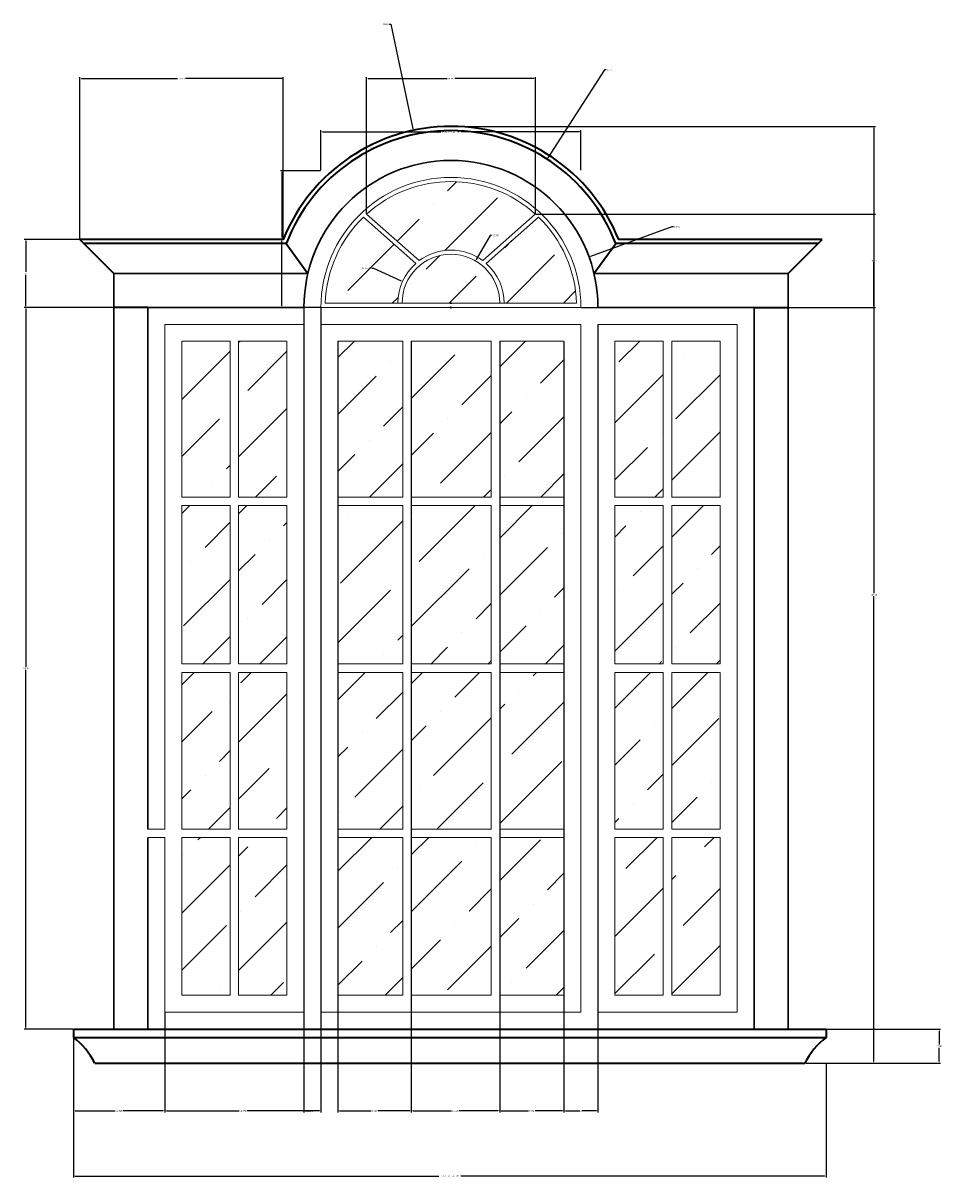
# Model space of a CAD drawing. Units: inches. Extents: x 386 to 708, y 151 to 489.
# Tile 3 of 4: x 386 to 494, y 353 to 489. Entities that reach past the tile are written whole.
import ezdxf

# ---------------------------------------------------------------- set-up
doc = ezdxf.new("R2010")
doc.units = ezdxf.units.IN
doc.header["$MEASUREMENT"] = 0
for name, color, linetype, lineweight in [('A-ANNO-DIMS', 2, 'Continuous', 18), ('A-GLAZ-FRAM', 4, 'Continuous', 30), ('A-GLAZ-PATT', 252, 'Continuous', 13), ('A-GLAZ-SASH', 4, 'Continuous', 18), ('A-GLAZ-SILL', 7, 'Continuous', 35), ('A-GLAZ-TRIM', 7, 'Continuous', 35)]:
    doc.layers.add(name, color=color, linetype=linetype, lineweight=lineweight)
doc.styles.get("Standard").update_dxf_attribs({"font": 'arial.ttf'})
doc.dimstyles.get("Standard").update_dxf_attribs({"dimtxt": 0.18, "dimasz": 0.18, "dimexe": 0.18, "dimexo": 0.0625, "dimgap": 0.09, "dimtad": 0, "dimtih": 1, "dimtoh": 1, "dimdec": 4, "dimzin": 0, "dimdsep": 46, "dimtxsty": 'Standard', "dimcen": 0.09, "dimadec": 0, "dimazin": 0, "dimtfac": 1, "dimtdec": 4, "dimtofl": 0, "dimtmove": 0, "dimatfit": 3, "dimfxl": 1, "dimtolj": 1, "dimtzin": 0, "dimarcsym": 0})

# ---------------------------------------------------------------- blocks, each defined once
blk = doc.blocks.new('WIN-SASH-2X4-L')
for p, q in [((9.69, 60.63), (9.69, 78.96)), ((10.69, 60.63), (10.69, 78.96)), ((4, 60.63), (9.69, 60.63)), ((10.69, 60.63), (16.38, 60.63)), ((4, 59.63), (9.69, 59.63)), ((9.69, 40.98), (9.69, 59.63)), ((10.69, 59.63), (16.38, 59.63)), ((10.69, 40.98), (10.69, 59.63)), ((4, 40.98), (9.69, 40.98)), ((10.69, 40.98), (16.38, 40.98)), ((4, 39.98), (9.69, 39.98)), ((9.69, 21.54), (9.69, 39.98)), ((10.69, 39.98), (16.38, 39.98)), ((10.69, 21.54), (10.69, 39.98)), ((0, 21.54), (2, 21.54)), ((0, 20.54), (2, 20.54)), ((4, 21.54), (9.69, 21.54)), ((4, 20.54), (9.69, 20.54)), ((9.69, 2), (9.69, 20.54)), ((10.69, 21.54), (16.38, 21.54)), ((10.69, 2), (10.69, 20.54)), ((10.69, 20.54), (16.38, 20.54))]:
    blk.add_line(p, q)
for points in [[(2, 20.54), (2, 0), (18.38, 0), (18.38, 80.96), (2, 80.96), (2, 21.54)], [(9.69, 78.96), (4, 78.96), (4, 60.63)], [(16.38, 60.63), (16.38, 78.96), (10.69, 78.96)], [(4, 59.63), (4, 40.98)], [(16.38, 40.98), (16.38, 59.63)], [(4, 39.98), (4, 21.54)], [(16.38, 21.54), (16.38, 39.98)], [(4, 20.54), (4, 2), (9.69, 2)], [(10.69, 2), (16.38, 2), (16.38, 20.54)]]:
    blk.add_lwpolyline(points)
blk = doc.blocks.new('WIN-SASH-2X4-R')
for p, q in [((7.69, 60.63), (7.69, 78.96)), ((8.69, 60.63), (8.69, 78.96)), ((2, 60.63), (7.69, 60.63)), ((8.69, 60.63), (14.38, 60.63)), ((2, 59.63), (7.69, 59.63)), ((7.69, 40.98), (7.69, 59.63)), ((8.69, 40.98), (8.69, 59.63)), ((8.69, 59.63), (14.38, 59.63)), ((2, 40.98), (7.69, 40.98)), ((8.69, 40.98), (14.38, 40.98)), ((2, 39.98), (7.69, 39.98)), ((7.69, 21.54), (7.69, 39.98)), ((8.69, 21.54), (8.69, 39.98)), ((8.69, 39.98), (14.38, 39.98)), ((2, 21.54), (7.69, 21.54)), ((2, 20.54), (7.69, 20.54)), ((7.69, 2), (7.69, 20.54)), ((8.69, 21.54), (14.38, 21.54)), ((8.69, 2), (8.69, 20.54)), ((8.69, 20.54), (14.38, 20.54))]:
    blk.add_line(p, q)
blk.add_lwpolyline([(0, 0), (16.38, 0), (16.38, 80.96), (0, 80.96)], close=True)
for points in [[(7.69, 78.96), (2, 78.96), (2, 60.63)], [(14.38, 60.63), (14.38, 78.96), (8.69, 78.96)], [(2, 59.63), (2, 40.98)], [(14.38, 40.98), (14.38, 59.63)], [(2, 39.98), (2, 21.54)], [(14.38, 21.54), (14.38, 39.98)], [(2, 20.54), (2, 2), (7.69, 2)], [(8.69, 2), (14.38, 2), (14.38, 20.54)]]:
    blk.add_lwpolyline(points)
blk = doc.blocks.new('WIN-SASH-3X4')
for p, q in [((9.62, 60.63), (9.62, 78.96)), ((10.62, 60.63), (10.62, 78.96)), ((20.04, 60.63), (20.04, 78.96)), ((21.04, 60.63), (21.04, 78.96)), ((2, 60.63), (9.62, 60.63)), ((10.62, 60.63), (20.04, 60.63)), ((21.04, 60.63), (28.6, 60.63)), ((21.04, 60.63), (28.6, 60.63)), ((2, 59.63), (9.62, 59.63)), ((9.62, 40.98), (9.62, 59.63)), ((10.62, 40.98), (10.62, 59.63)), ((10.62, 59.63), (20.04, 59.63)), ((20.04, 40.98), (20.04, 59.63)), ((21.04, 59.63), (28.6, 59.63)), ((21.04, 40.98), (21.04, 59.63)), ((21.04, 59.63), (28.6, 59.63)), ((2, 40.98), (9.62, 40.98)), ((10.62, 40.98), (20.04, 40.98)), ((21.04, 40.98), (28.6, 40.98)), ((21.04, 40.98), (28.6, 40.98)), ((2, 39.98), (9.62, 39.98)), ((9.62, 21.54), (9.62, 39.98)), ((10.62, 21.54), (10.62, 39.98)), ((10.62, 39.98), (20.04, 39.98)), ((20.04, 21.54), (20.04, 39.98)), ((21.04, 39.98), (28.6, 39.98)), ((21.04, 21.54), (21.04, 39.98)), ((21.04, 39.98), (28.6, 39.98)), ((2, 21.54), (9.62, 21.54)), ((2, 20.54), (9.62, 20.54)), ((9.62, 2), (9.62, 20.54)), ((10.62, 21.54), (20.04, 21.54)), ((10.62, 2), (10.62, 20.54)), ((10.62, 20.54), (20.04, 20.54)), ((20.04, 2), (20.04, 20.54)), ((21.04, 21.54), (28.6, 21.54)), ((21.04, 21.54), (28.6, 21.54)), ((21.04, 2), (21.04, 20.54)), ((21.04, 20.54), (28.6, 20.54)), ((21.04, 20.54), (28.6, 20.54))]:
    blk.add_line(p, q)
blk.add_lwpolyline([(30.6, 0), (30.6, 80.96), (0, 80.96), (0, 0)], close=True)
for points in [[(9.62, 78.96), (2, 78.96), (2, 60.63)], [(20.04, 78.96), (10.62, 78.96)], [(28.6, 60.63), (28.6, 78.96), (21.04, 78.96)], [(2, 59.63), (2, 40.98)], [(28.6, 40.98), (28.6, 59.63)], [(2, 39.98), (2, 21.54)], [(28.6, 21.54), (28.6, 39.98)], [(2, 20.54), (2, 2), (9.62, 2)], [(21.04, 2), (28.6, 2), (28.6, 20.54)], [(10.62, 2), (20.04, 2)]]:
    blk.add_lwpolyline(points)
blk = doc.blocks.new('WIN-FANLIGHT-RADIAL')
for p, q in [((11.55, 5.5), (5.37, 10.98)), ((19.05, 5.5), (25.23, 10.98)), ((11.16, 5.18), (5.01, 10.63)), ((19.44, 5.18), (25.6, 10.63))]:
    blk.add_line(p, q)
blk.add_lwpolyline([(30.6, 0), (0, 0, -1)], format="xyb", close=True)
for points in [[(5.37, 10.98, -0.385138), (25.23, 10.98, -0.385138)], [(25.6, 10.63, -0.194348), (30.09, 0.5), (0.51, 0.5, -0.194348), (5.01, 10.63)]]:
    blk.add_lwpolyline(points, format="xyb")
for radius, start, end in [(5.75, 0, 180), (6.25, 53.1161, 126.8839), (6.25, 131.5309, 180), (6.25, 0, 48.4691)]:
    blk.add_arc((15.3, 0.5), radius, start, end)
blk = doc.blocks.new('WIN-SILL-TRIPLE')
for p, q in [((0, 4), (88.59, 4)), ((0, 4), (0, 3)), ((0, 3), (88.59, 3)), ((88.59, 4), (88.59, 3)), ((2.5, 0), (86.09, 0))]:
    blk.add_line(p, q)
blk.add_lwpolyline([(4.75, 0), (84.1, 0)])
for centre, start, end in [((-4.74, -3.48), 25.6893, 53.8074), ((93.33, -3.48), 126.1926, 154.3107)]:
    blk.add_arc(centre, 8.03, start, end)
blk = doc.blocks.new('*D14')
at = {"layer": 'A-ANNO-DIMS', "color": 0, "lineweight": -2, "transparency": 16777216}
for p, q in [((420.9, 471.8), (420.9, 476.5)), ((421.08, 476.32), (435.02, 476.32)), ((451.32, 476.32), (437.38, 476.32)), ((451.5, 471.8), (451.5, 476.5))]:
    blk.add_line(p, q, dxfattribs=at)
at = {"layer": 'A-ANNO-DIMS', "color": 0, "transparency": 16777216}
for points in [[(421.08, 476.35), (421.08, 476.29), (420.9, 476.32)], [(451.32, 476.35), (451.32, 476.29), (451.5, 476.32)]]:
    blk.add_solid(points, dxfattribs=at)
at = {"layer": 'Defpoints', "color": 0, "transparency": 16777216}
for p in [(451.5, 476.32), (420.9, 471.73), (451.5, 471.73)]:
    blk.add_point(p, dxfattribs=at)
at = {"layer": 'A-ANNO-DIMS', "color": 0, "transparency": 16777216, "insert": (436.2, 476.32), "char_height": 0.18, "attachment_point": 5}
blk.add_mtext('\\A1;FANLIGHT 31 TYP.', dxfattribs=at)
blk = doc.blocks.new('*D15')
at = {"layer": 'A-ANNO-DIMS', "color": 0, "lineweight": -2, "transparency": 16777216}
for p, q in [((420.83, 471.73), (416.13, 471.73)), ((416.31, 471.55), (416.31, 463.88)), ((416.31, 455.84), (416.31, 463.51)), ((420.83, 455.66), (416.13, 455.66))]:
    blk.add_line(p, q, dxfattribs=at)
at = {"layer": 'A-ANNO-DIMS', "color": 0, "transparency": 16777216}
for points in [[(416.28, 471.55), (416.34, 471.55), (416.31, 471.73)], [(416.28, 455.84), (416.34, 455.84), (416.31, 455.66)]]:
    blk.add_solid(points, dxfattribs=at)
at = {"layer": 'Defpoints', "color": 0, "transparency": 16777216}
for p in [(416.31, 471.73), (420.9, 471.73), (420.9, 455.66)]:
    blk.add_point(p, dxfattribs=at)
at = {"layer": 'A-ANNO-DIMS', "color": 0, "transparency": 16777216, "insert": (416.31, 463.7), "char_height": 0.18, "attachment_point": 5}
blk.add_mtext('\\A1;16 TYP.', dxfattribs=at)
blk = doc.blocks.new('*D16')
at = {"layer": 'A-ANNO-DIMS', "color": 0, "lineweight": -2, "transparency": 16777216}
for p, q in [((391.77, 366.64), (391.77, 353.23)), ((480.36, 366.64), (480.36, 353.23)), ((391.95, 353.41), (434.77, 353.41)), ((480.18, 353.41), (437.37, 353.41))]:
    blk.add_line(p, q, dxfattribs=at)
at = {"layer": 'A-ANNO-DIMS', "color": 0, "transparency": 16777216}
for points in [[(391.95, 353.44), (391.95, 353.38), (391.77, 353.41)], [(480.18, 353.44), (480.18, 353.38), (480.36, 353.41)]]:
    blk.add_solid(points, dxfattribs=at)
at = {"layer": 'Defpoints', "color": 0, "transparency": 16777216}
for p in [(391.77, 366.7), (480.36, 366.7), (480.36, 353.41)]:
    blk.add_point(p, dxfattribs=at)
at = {"layer": 'A-ANNO-DIMS', "color": 0, "transparency": 16777216, "insert": (436.07, 353.41), "char_height": 0.18, "attachment_point": 5}
blk.add_mtext('\\A1;TRIPLE SILL 89 TYP.', dxfattribs=at)
blk = doc.blocks.new('*D17')
at = {"layer": 'A-ANNO-DIMS', "color": 0, "lineweight": -2, "transparency": 16777216}
for p, q in [((480.42, 370.7), (493.83, 370.7)), ((493.65, 370.52), (493.65, 368.88)), ((493.65, 366.88), (493.65, 368.52)), ((480.42, 366.7), (493.83, 366.7))]:
    blk.add_line(p, q, dxfattribs=at)
at = {"layer": 'A-ANNO-DIMS', "color": 0, "transparency": 16777216}
for points in [[(493.62, 370.52), (493.68, 370.52), (493.65, 370.7)], [(493.62, 366.88), (493.68, 366.88), (493.65, 366.7)]]:
    blk.add_solid(points, dxfattribs=at)
at = {"layer": 'Defpoints', "color": 0, "transparency": 16777216}
for p in [(480.36, 370.7), (493.65, 370.7), (480.36, 366.7)]:
    blk.add_point(p, dxfattribs=at)
at = {"layer": 'A-ANNO-DIMS', "color": 0, "transparency": 16777216, "insert": (493.65, 368.7), "char_height": 0.18, "attachment_point": 5}
blk.add_mtext('\\A1;4 TYP.', dxfattribs=at)
blk = doc.blocks.new('*D22')
at = {"layer": 'A-ANNO-DIMS', "color": 0, "lineweight": -2, "transparency": 16777216}
for p, q in [((436.26, 476.96), (486.16, 476.96)), ((485.98, 476.78), (485.98, 422.01)), ((485.98, 366.88), (485.98, 421.65)), ((477.93, 366.7), (486.16, 366.7))]:
    blk.add_line(p, q, dxfattribs=at)
at = {"layer": 'A-ANNO-DIMS', "color": 0, "transparency": 16777216}
for points in [[(485.95, 476.78), (486.01, 476.78), (485.98, 476.96)], [(485.95, 366.88), (486.01, 366.88), (485.98, 366.7)]]:
    blk.add_solid(points, dxfattribs=at)
at = {"layer": 'Defpoints', "color": 0, "transparency": 16777216}
for p in [(436.2, 476.96), (485.98, 476.96), (477.87, 366.7)]:
    blk.add_point(p, dxfattribs=at)
at = {"layer": 'A-ANNO-DIMS', "color": 0, "transparency": 16777216, "insert": (485.98, 421.83), "char_height": 0.18, "attachment_point": 5}
blk.add_mtext('\\A1;110.26', dxfattribs=at)
blk = doc.blocks.new('*D23')
at = {"layer": 'A-ANNO-DIMS', "color": 0, "lineweight": -2, "transparency": 16777216}
for p, q in [((418.83, 455.66), (385.97, 455.66)), ((386.15, 455.48), (386.15, 413.36)), ((386.15, 370.88), (386.15, 413)), ((391.71, 370.7), (385.97, 370.7))]:
    blk.add_line(p, q, dxfattribs=at)
at = {"layer": 'A-ANNO-DIMS', "color": 0, "transparency": 16777216}
for points in [[(386.12, 455.48), (386.18, 455.48), (386.15, 455.66)], [(386.12, 370.88), (386.18, 370.88), (386.15, 370.7)]]:
    blk.add_solid(points, dxfattribs=at)
at = {"layer": 'Defpoints', "color": 0, "transparency": 16777216}
for p in [(386.15, 455.66), (418.9, 455.66), (391.77, 370.7)]:
    blk.add_point(p, dxfattribs=at)
at = {"layer": 'A-ANNO-DIMS', "color": 0, "transparency": 16777216, "insert": (386.15, 413.18), "char_height": 0.18, "attachment_point": 5}
blk.add_mtext('\\A1;84.96', dxfattribs=at)
blk = doc.blocks.new('*D24')
at = {"layer": 'A-ANNO-DIMS', "color": 0, "lineweight": -2, "transparency": 16777216}
for p, q in [((392.52, 463.72), (392.52, 482.76)), ((392.7, 482.58), (404.02, 482.58)), ((416.28, 482.58), (404.95, 482.58)), ((416.46, 463.72), (416.46, 482.76))]:
    blk.add_line(p, q, dxfattribs=at)
at = {"layer": 'A-ANNO-DIMS', "color": 0, "transparency": 16777216}
for points in [[(392.7, 482.61), (392.7, 482.55), (392.52, 482.58)], [(416.28, 482.61), (416.28, 482.55), (416.46, 482.58)]]:
    blk.add_solid(points, dxfattribs=at)
at = {"layer": 'Defpoints', "color": 0, "transparency": 16777216}
for p in [(416.46, 482.58), (392.52, 463.66), (416.46, 463.66)]:
    blk.add_point(p, dxfattribs=at)
at = {"layer": 'A-ANNO-DIMS', "color": 0, "transparency": 16777216, "insert": (404.49, 482.58), "char_height": 0.18, "attachment_point": 5}
blk.add_mtext('\\A1;23.937', dxfattribs=at)
blk = doc.blocks.new('*D25')
at = {"layer": 'A-ANNO-DIMS', "color": 0, "lineweight": -2, "transparency": 16777216}
for p, q in [((402.52, 372.64), (402.52, 360.9)), ((391.77, 370.64), (391.77, 360.9)), ((391.95, 361.08), (396.69, 361.08)), ((402.34, 361.08), (397.6, 361.08))]:
    blk.add_line(p, q, dxfattribs=at)
at = {"layer": 'A-ANNO-DIMS', "color": 0, "transparency": 16777216}
for points in [[(391.95, 361.11), (391.95, 361.05), (391.77, 361.08)], [(402.34, 361.11), (402.34, 361.05), (402.52, 361.08)]]:
    blk.add_solid(points, dxfattribs=at)
at = {"layer": 'Defpoints', "color": 0, "transparency": 16777216}
for p in [(402.52, 372.7), (391.77, 370.7), (402.52, 361.08)]:
    blk.add_point(p, dxfattribs=at)
at = {"layer": 'A-ANNO-DIMS', "color": 0, "transparency": 16777216, "insert": (397.15, 361.08), "char_height": 0.18, "attachment_point": 5}
blk.add_mtext('\\A1;10.746', dxfattribs=at)
blk = doc.blocks.new('*D26')
at = {"layer": 'A-ANNO-DIMS', "color": 0, "lineweight": -2, "transparency": 16777216}
for p, q in [((402.52, 372.64), (402.52, 360.9)), ((420.9, 372.64), (420.9, 360.9)), ((402.7, 361.08), (411.25, 361.08)), ((420.72, 361.08), (412.16, 361.08))]:
    blk.add_line(p, q, dxfattribs=at)
at = {"layer": 'A-ANNO-DIMS', "color": 0, "transparency": 16777216}
for points in [[(402.7, 361.11), (402.7, 361.05), (402.52, 361.08)], [(420.72, 361.11), (420.72, 361.05), (420.9, 361.08)]]:
    blk.add_solid(points, dxfattribs=at)
at = {"layer": 'Defpoints', "color": 0, "transparency": 16777216}
for p in [(402.52, 372.7), (420.9, 372.7), (420.9, 361.08)]:
    blk.add_point(p, dxfattribs=at)
at = {"layer": 'A-ANNO-DIMS', "color": 0, "transparency": 16777216, "insert": (411.71, 361.08), "char_height": 0.18, "attachment_point": 5}
blk.add_mtext('\\A1;18.378', dxfattribs=at)
blk = doc.blocks.new('*D27')
at = {"layer": 'A-ANNO-DIMS', "color": 0, "lineweight": -2, "transparency": 16777216}
for p, q in [((422.9, 451.6), (422.9, 360.9)), ((431.52, 451.6), (431.52, 360.9)), ((423.08, 361.08), (426.81, 361.08)), ((431.34, 361.08), (427.6, 361.08))]:
    blk.add_line(p, q, dxfattribs=at)
at = {"layer": 'A-ANNO-DIMS', "color": 0, "transparency": 16777216}
for points in [[(423.08, 361.11), (423.08, 361.05), (422.9, 361.08)], [(431.34, 361.11), (431.34, 361.05), (431.52, 361.08)]]:
    blk.add_solid(points, dxfattribs=at)
at = {"layer": 'Defpoints', "color": 0, "transparency": 16777216}
for p in [(422.9, 451.66), (431.52, 451.66), (431.52, 361.08)]:
    blk.add_point(p, dxfattribs=at)
at = {"layer": 'A-ANNO-DIMS', "color": 0, "transparency": 16777216, "insert": (427.21, 361.08), "char_height": 0.18, "attachment_point": 5}
blk.add_mtext('\\A1;8.618', dxfattribs=at)
blk = doc.blocks.new('*D28')
at = {"layer": 'A-ANNO-DIMS', "color": 0, "lineweight": -2, "transparency": 16777216}
for p, q in [((431.52, 451.6), (431.52, 360.9)), ((441.94, 451.6), (441.94, 360.9)), ((431.7, 361.08), (436.27, 361.08)), ((441.76, 361.08), (437.18, 361.08))]:
    blk.add_line(p, q, dxfattribs=at)
at = {"layer": 'A-ANNO-DIMS', "color": 0, "transparency": 16777216}
for points in [[(431.7, 361.11), (431.7, 361.05), (431.52, 361.08)], [(441.76, 361.11), (441.76, 361.05), (441.94, 361.08)]]:
    blk.add_solid(points, dxfattribs=at)
at = {"layer": 'Defpoints', "color": 0, "transparency": 16777216}
for p in [(431.52, 451.66), (441.94, 451.66), (441.94, 361.08)]:
    blk.add_point(p, dxfattribs=at)
at = {"layer": 'A-ANNO-DIMS', "color": 0, "transparency": 16777216, "insert": (436.73, 361.08), "char_height": 0.18, "attachment_point": 5}
blk.add_mtext('\\A1;10.423', dxfattribs=at)
blk = doc.blocks.new('*D29')
at = {"layer": 'A-ANNO-DIMS', "color": 0, "lineweight": -2, "transparency": 16777216}
for p, q in [((441.94, 451.6), (441.94, 360.9)), ((449.5, 451.6), (449.5, 360.9)), ((442.12, 361.08), (445.34, 361.08)), ((449.32, 361.08), (446.09, 361.08))]:
    blk.add_line(p, q, dxfattribs=at)
at = {"layer": 'A-ANNO-DIMS', "color": 0, "transparency": 16777216}
for points in [[(442.12, 361.11), (442.12, 361.05), (441.94, 361.08)], [(449.32, 361.11), (449.32, 361.05), (449.5, 361.08)]]:
    blk.add_solid(points, dxfattribs=at)
at = {"layer": 'Defpoints', "color": 0, "transparency": 16777216}
for p in [(441.94, 451.66), (449.5, 451.66), (449.5, 361.08)]:
    blk.add_point(p, dxfattribs=at)
at = {"layer": 'A-ANNO-DIMS', "color": 0, "transparency": 16777216, "insert": (445.72, 361.08), "char_height": 0.18, "attachment_point": 5}
blk.add_mtext('\\A1;7.561', dxfattribs=at)
blk = doc.blocks.new('*D30')
at = {"layer": 'A-ANNO-DIMS', "color": 0, "lineweight": -2, "transparency": 16777216}
for p, q in [((453.5, 453.6), (453.5, 360.9)), ((449.5, 451.6), (449.5, 360.9)), ((449.68, 361.08), (451.35, 361.08)), ((453.32, 361.08), (451.65, 361.08))]:
    blk.add_line(p, q, dxfattribs=at)
at = {"layer": 'A-ANNO-DIMS', "color": 0, "transparency": 16777216}
for points in [[(449.68, 361.11), (449.68, 361.05), (449.5, 361.08)], [(453.32, 361.11), (453.32, 361.05), (453.5, 361.08)]]:
    blk.add_solid(points, dxfattribs=at)
at = {"layer": 'Defpoints', "color": 0, "transparency": 16777216}
for p in [(453.5, 453.66), (449.5, 451.66), (453.5, 361.08)]:
    blk.add_point(p, dxfattribs=at)
at = {"layer": 'A-ANNO-DIMS', "color": 0, "transparency": 16777216, "insert": (451.5, 361.08), "char_height": 0.18, "attachment_point": 5}
blk.add_mtext('\\A1;4', dxfattribs=at)
blk = doc.blocks.new('*D31')
at = {"layer": 'A-ANNO-DIMS', "color": 0, "lineweight": -2, "transparency": 16777216}
for p, q in [((392.46, 463.66), (385.97, 463.66)), ((386.15, 463.48), (386.15, 459.84)), ((386.15, 455.84), (386.15, 459.48)), ((418.83, 455.66), (385.97, 455.66))]:
    blk.add_line(p, q, dxfattribs=at)
at = {"layer": 'A-ANNO-DIMS', "color": 0, "transparency": 16777216}
for points in [[(386.12, 463.48), (386.18, 463.48), (386.15, 463.66)], [(386.12, 455.84), (386.18, 455.84), (386.15, 455.66)]]:
    blk.add_solid(points, dxfattribs=at)
at = {"layer": 'Defpoints', "color": 0, "transparency": 16777216}
for p in [(386.15, 463.66), (392.52, 463.66), (418.9, 455.66)]:
    blk.add_point(p, dxfattribs=at)
at = {"layer": 'A-ANNO-DIMS', "color": 0, "transparency": 16777216, "insert": (386.15, 459.66), "char_height": 0.18, "attachment_point": 5}
blk.add_mtext('\\A1;8', dxfattribs=at)
blk = doc.blocks.new('*D32')
at = {"layer": 'A-ANNO-DIMS', "color": 0, "lineweight": -2, "transparency": 16777216}
for p, q in [((418.9, 455.6), (418.9, 360.9)), ((420.9, 455.6), (420.9, 360.9)), ((419.08, 361.08), (419.75, 361.08)), ((420.72, 361.08), (420.05, 361.08))]:
    blk.add_line(p, q, dxfattribs=at)
at = {"layer": 'A-ANNO-DIMS', "color": 0, "transparency": 16777216}
for points in [[(419.08, 361.11), (419.08, 361.05), (418.9, 361.08)], [(420.72, 361.11), (420.72, 361.05), (420.9, 361.08)]]:
    blk.add_solid(points, dxfattribs=at)
at = {"layer": 'Defpoints', "color": 0, "transparency": 16777216}
for p in [(418.9, 455.66), (420.9, 455.66), (420.9, 361.08)]:
    blk.add_point(p, dxfattribs=at)
at = {"layer": 'A-ANNO-DIMS', "color": 0, "transparency": 16777216, "insert": (419.9, 361.08), "char_height": 0.18, "attachment_point": 5}
blk.add_mtext('\\A1;2', dxfattribs=at)
blk = doc.blocks.new('*D33')
at = {"layer": 'A-ANNO-DIMS', "color": 0, "lineweight": -2, "transparency": 16777216}
for p, q in [((426.27, 466.7), (426.27, 482.76)), ((426.45, 482.58), (435.74, 482.58)), ((445.95, 482.58), (436.65, 482.58)), ((446.13, 466.7), (446.13, 482.76))]:
    blk.add_line(p, q, dxfattribs=at)
at = {"layer": 'A-ANNO-DIMS', "color": 0, "transparency": 16777216}
for points in [[(426.45, 482.61), (426.45, 482.55), (426.27, 482.58)], [(445.95, 482.61), (445.95, 482.55), (446.13, 482.58)]]:
    blk.add_solid(points, dxfattribs=at)
at = {"layer": 'Defpoints', "color": 0, "transparency": 16777216}
for p in [(446.13, 482.58), (426.27, 466.64), (446.13, 466.64)]:
    blk.add_point(p, dxfattribs=at)
at = {"layer": 'A-ANNO-DIMS', "color": 0, "transparency": 16777216, "insert": (436.2, 482.58), "char_height": 0.18, "attachment_point": 5}
blk.add_mtext('\\A1;19.857', dxfattribs=at)
blk = doc.blocks.new('*D34')
at = {"layer": 'A-ANNO-DIMS', "color": 0, "lineweight": -2, "transparency": 16777216}
for p, q in [((446.19, 466.64), (486.16, 466.64)), ((485.98, 466.46), (485.98, 461.33)), ((485.98, 455.84), (485.98, 460.96)), ((451.56, 455.66), (486.16, 455.66))]:
    blk.add_line(p, q, dxfattribs=at)
at = {"layer": 'A-ANNO-DIMS', "color": 0, "transparency": 16777216}
for points in [[(485.95, 466.46), (486.01, 466.46), (485.98, 466.64)], [(485.95, 455.84), (486.01, 455.84), (485.98, 455.66)]]:
    blk.add_solid(points, dxfattribs=at)
at = {"layer": 'Defpoints', "color": 0, "transparency": 16777216}
for p in [(446.13, 466.64), (485.98, 466.64), (451.5, 455.66)]:
    blk.add_point(p, dxfattribs=at)
at = {"layer": 'A-ANNO-DIMS', "color": 0, "transparency": 16777216, "insert": (485.98, 461.15), "char_height": 0.18, "attachment_point": 5}
blk.add_mtext('\\A1;10.977', dxfattribs=at)
blk = doc.blocks.new('*D78')
at = {"layer": 'A-ANNO-DIMS', "color": 0, "lineweight": -2, "transparency": 16777216}
for p, q in [((428.93, 488.99), (429.11, 488.99)), ((429.11, 488.99), (431.73, 476.67)), ((436.11, 455.66), (436.29, 455.66)), ((436.2, 455.57), (436.2, 455.75))]:
    blk.add_line(p, q, dxfattribs=at)
at = {"layer": 'A-ANNO-DIMS', "color": 0, "transparency": 16777216}
blk.add_solid([(431.76, 476.68), (431.7, 476.66), (431.77, 476.49)], dxfattribs=at)
at = {"layer": 'Defpoints', "color": 0, "transparency": 16777216}
for p in [(431.77, 476.49), (436.2, 455.66)]:
    blk.add_point(p, dxfattribs=at)
at = {"layer": 'A-ANNO-DIMS', "color": 0, "transparency": 16777216, "insert": (428.52, 488.99), "char_height": 0.18, "attachment_point": 5}
blk.add_mtext('\\A1;R21.3', dxfattribs=at)
blk = doc.blocks.new('*D79')
at = {"layer": 'A-ANNO-DIMS', "color": 0, "lineweight": -2, "transparency": 16777216}
for p, q in [((454.28, 483.6), (447.6, 473.27)), ((454.46, 483.6), (454.28, 483.6)), ((436.11, 455.66), (436.29, 455.66)), ((436.2, 455.57), (436.2, 455.75))]:
    blk.add_line(p, q, dxfattribs=at)
at = {"layer": 'A-ANNO-DIMS', "color": 0, "transparency": 16777216}
blk.add_solid([(447.57, 473.29), (447.62, 473.26), (447.5, 473.12)], dxfattribs=at)
at = {"layer": 'Defpoints', "color": 0, "transparency": 16777216}
for p in [(447.5, 473.12), (436.2, 455.66)]:
    blk.add_point(p, dxfattribs=at)
at = {"layer": 'A-ANNO-DIMS', "color": 0, "transparency": 16777216, "insert": (454.87, 483.6), "char_height": 0.18, "attachment_point": 5}
blk.add_mtext('\\A1;R20.8', dxfattribs=at)
blk = doc.blocks.new('*D80')
at = {"layer": 'A-ANNO-DIMS', "color": 0, "lineweight": -2, "transparency": 16777216}
for p, q in [((462.21, 465.13), (452.63, 461.64)), ((462.39, 465.13), (462.21, 465.13)), ((436.11, 455.66), (436.29, 455.66)), ((436.2, 455.57), (436.2, 455.75))]:
    blk.add_line(p, q, dxfattribs=at)
at = {"layer": 'A-ANNO-DIMS', "color": 0, "transparency": 16777216}
blk.add_solid([(452.61, 461.67), (452.64, 461.61), (452.46, 461.58)], dxfattribs=at)
at = {"layer": 'Defpoints', "color": 0, "transparency": 16777216}
for p in [(452.46, 461.58), (436.2, 455.66)]:
    blk.add_point(p, dxfattribs=at)
at = {"layer": 'A-ANNO-DIMS', "color": 0, "transparency": 16777216, "insert": (462.8, 465.13), "char_height": 0.18, "attachment_point": 5}
blk.add_mtext('\\A1;R17.3', dxfattribs=at)
blk = doc.blocks.new('*D81')
at = {"layer": 'A-ANNO-DIMS', "color": 0, "lineweight": -2, "transparency": 16777216}
for p, q in [((426.9, 460.26), (427.08, 460.26)), ((427.08, 460.26), (430.34, 458.8)), ((436.11, 456.16), (436.29, 456.16)), ((436.2, 456.07), (436.2, 456.25))]:
    blk.add_line(p, q, dxfattribs=at)
at = {"layer": 'A-ANNO-DIMS', "color": 0, "transparency": 16777216}
blk.add_solid([(430.35, 458.82), (430.33, 458.77), (430.5, 458.72)], dxfattribs=at)
at = {"layer": 'Defpoints', "color": 0, "transparency": 16777216}
for p in [(430.5, 458.72), (436.2, 456.16)]:
    blk.add_point(p, dxfattribs=at)
at = {"layer": 'A-ANNO-DIMS', "color": 0, "transparency": 16777216, "insert": (426.23, 460.26), "char_height": 0.18, "attachment_point": 5}
blk.add_mtext('\\A1;3X R6.247', dxfattribs=at)
blk = doc.blocks.new('*D82')
at = {"layer": 'A-ANNO-DIMS', "color": 0, "lineweight": -2, "transparency": 16777216}
for p, q in [((440.8, 464.12), (439.16, 461.29)), ((440.98, 464.12), (440.8, 464.12)), ((436.11, 456.16), (436.29, 456.16)), ((436.2, 456.07), (436.2, 456.25))]:
    blk.add_line(p, q, dxfattribs=at)
at = {"layer": 'A-ANNO-DIMS', "color": 0, "transparency": 16777216}
blk.add_solid([(439.14, 461.31), (439.19, 461.28), (439.07, 461.13)], dxfattribs=at)
at = {"layer": 'Defpoints', "color": 0, "transparency": 16777216}
for p in [(439.07, 461.13), (436.2, 456.16)]:
    blk.add_point(p, dxfattribs=at)
at = {"layer": 'A-ANNO-DIMS', "color": 0, "transparency": 16777216, "insert": (441.46, 464.12), "char_height": 0.18, "attachment_point": 5}
blk.add_mtext('\\A1;R5.747', dxfattribs=at)

msp = doc.modelspace()

# ---------------------------------------------------------------- hatches: boundary and pattern name
at = {"layer": 'A-GLAZ-PATT'}
h = msp.add_hatch(dxfattribs=at)
h.set_pattern_fill('ANSI36', color=256, scale=38)
h.paths.add_polyline_path([(432.0564, 460.8344, 0.21469693), (429.9512, 456.1577), (430.4512, 456.1577, -1), (441.9457, 456.1577), (442.4457, 456.1577, 0.21469693), (440.3405, 460.8344), (446.4934, 466.2919, -0.19434814), (450.9912, 456.1577), (421.4058, 456.1577, -0.19434814), (425.9035, 466.2919)])
h.paths.add_polyline_path([(446.1268, 466.6351, 0.38513823), (426.2702, 466.6351), (432.4489, 461.1546, -0.33346908), (439.948, 461.1546)])
h.paths.add_polyline_path([(461.1886, 451.6577), (455.4996, 451.6577), (455.4996, 433.3276), (461.1886, 433.3276)])
h.paths.add_polyline_path([(467.8775, 451.6577), (462.1886, 451.6577), (462.1886, 433.3276), (467.8775, 433.3276)])
h.paths.add_polyline_path([(449.4996, 451.6577), (441.9385, 451.6577), (441.9385, 433.3276), (449.4996, 433.3276)])
h.paths.add_polyline_path([(440.9385, 451.6577), (431.5153, 451.6577), (431.5153, 433.3276), (440.9385, 433.3276)])
h.paths.add_polyline_path([(430.5153, 451.6577), (422.8973, 451.6577), (422.8973, 433.3276), (430.5153, 433.3276)])
h.paths.add_polyline_path([(416.8973, 451.6577), (411.2084, 451.6577), (411.2084, 433.3276), (416.8973, 433.3276)])
h.paths.add_polyline_path([(410.2084, 451.6577), (404.5194, 451.6577), (404.5194, 433.3276), (410.2084, 433.3276)])
h.paths.add_polyline_path([(410.2084, 432.3276), (404.5194, 432.3276), (404.5194, 413.6799), (410.2084, 413.6799)])
h.paths.add_polyline_path([(416.8973, 432.3276), (411.2084, 432.3276), (411.2084, 413.6799), (416.8973, 413.6799)])
h.paths.add_polyline_path([(430.5153, 432.3276), (422.8973, 432.3276), (422.8973, 413.6799), (430.5153, 413.6799)])
h.paths.add_polyline_path([(440.9385, 432.3276), (431.5153, 432.3276), (431.5153, 413.6799), (440.9385, 413.6799)])
h.paths.add_polyline_path([(449.4996, 432.3276), (441.9385, 432.3276), (441.9385, 413.6799), (449.4996, 413.6799)])
h.paths.add_polyline_path([(461.1886, 432.3276), (455.4996, 432.3276), (455.4996, 413.6799), (461.1886, 413.6799)])
h.paths.add_polyline_path([(467.8775, 432.3276), (462.1886, 432.3276), (462.1886, 413.6799), (467.8775, 413.6799)])
h.paths.add_polyline_path([(467.8775, 412.6799), (462.1886, 412.6799), (462.1886, 394.239), (467.8775, 394.239)])
h.paths.add_polyline_path([(461.1886, 412.6799), (455.4996, 412.6799), (455.4996, 394.239), (461.1886, 394.239)])
h.paths.add_polyline_path([(449.4996, 412.6799), (441.9385, 412.6799), (441.9385, 394.239), (449.4996, 394.239)])
h.paths.add_polyline_path([(440.9385, 412.6799), (431.5153, 412.6799), (431.5153, 394.239), (440.9385, 394.239)])
h.paths.add_polyline_path([(430.5153, 412.6799), (422.8973, 412.6799), (422.8973, 394.239), (430.5153, 394.239)])
h.paths.add_polyline_path([(416.8973, 412.6799), (411.2084, 412.6799), (411.2084, 394.239), (416.8973, 394.239)])
h.paths.add_polyline_path([(410.2084, 412.6799), (404.5194, 412.6799), (404.5194, 394.239), (410.2084, 394.239)])
h.paths.add_polyline_path([(410.2084, 393.239), (404.5194, 393.239), (404.5194, 374.702), (410.2084, 374.702)])
h.paths.add_polyline_path([(416.8973, 393.239), (411.2084, 393.239), (411.2084, 374.702), (416.8973, 374.702)])
h.paths.add_polyline_path([(430.5153, 393.239), (422.8973, 393.239), (422.8973, 374.702), (430.5153, 374.702)])
h.paths.add_polyline_path([(440.9385, 393.239), (431.5153, 393.239), (431.5153, 374.702), (440.9385, 374.702)])
h.paths.add_polyline_path([(449.4996, 393.239), (441.9385, 393.239), (441.9385, 374.702), (449.4996, 374.702)])
h.paths.add_polyline_path([(461.1886, 393.239), (455.4996, 393.239), (455.4996, 374.702), (461.1886, 374.702)])
h.paths.add_polyline_path([(467.8775, 393.239), (462.1886, 393.239), (462.1886, 374.702), (467.8775, 374.702)])

# ---------------------------------------------------------------- linework, layer by layer
at = {"layer": 'A-GLAZ-FRAM'}
for points in [[(419.3661, 459.6577), (396.5194, 459.6577), (396.5194, 370.702)], [(475.8775, 370.702), (475.8775, 459.6577), (453.0309, 459.6577)], [(418.8973, 455.6577), (400.5194, 455.6577), (400.5194, 394.239)], [(400.5194, 393.239), (400.5194, 370.702), (471.8775, 370.702), (471.8775, 455.6577), (453.4996, 455.6577)]]:
    msp.add_lwpolyline(points, dxfattribs=at)
msp.add_arc((436.1985, 455.6577), 17.3011, 0, 180, dxfattribs=at)
at = {"layer": 'A-GLAZ-TRIM'}
for p, q in [((396.5194, 459.6577), (392.5194, 463.6577)), ((475.8775, 459.6577), (479.8775, 463.6577)), ((416.8048, 463.1791), (419.3661, 459.6577)), ((453.0309, 459.6577), (455.5922, 463.1791)), ((400.5194, 455.6577), (396.5194, 455.6577)), ((471.8775, 455.6577), (475.8775, 455.6577))]:
    msp.add_line(p, q, dxfattribs=at)
for points in [[(479.8775, 463.6577), (455.9403, 463.6577, 0.67375527), (416.4567, 463.6577), (392.5194, 463.6577)], [(479.3775, 463.1577), (455.6005, 463.1577, 0.68555526), (416.7965, 463.1577), (393.0194, 463.1577)]]:
    msp.add_lwpolyline(points, format="xyb", dxfattribs=at)

# ---------------------------------------------------------------- block references
at = {"layer": 'A-GLAZ-SASH'}
for name, p in [('WIN-FANLIGHT-RADIAL', (420.897, 455.658)), ('WIN-SASH-2X4-L', (400.519, 372.702)), ('WIN-SASH-3X4', (420.897, 372.702)), ('WIN-SASH-2X4-R', (453.5, 372.702))]:
    msp.add_blockref(name, p, dxfattribs=at)
at = {"layer": 'A-GLAZ-SILL'}
msp.add_blockref('WIN-SILL-TRIPLE', (391.773, 366.702), dxfattribs=at)

# ---------------------------------------------------------------- dimensions: what is measured, and where the dimension line sits
at = {"layer": 'A-ANNO-DIMS'}
for center, mpoint, override, picture, middle in [((436.1985, 455.6577), (431.7695, 476.4933), {"dimdec": 1, "dimlfac": 1, "dimrnd": 0, "dimzin": 0, "dimdsep": 46, "dimlunit": 2}, '*D78', (428.5222, 488.9947)), ((436.1985, 455.6577), (447.4995, 473.1212), {"dimdec": 1, "dimlfac": 1, "dimrnd": 0, "dimzin": 0, "dimdsep": 46, "dimlunit": 2}, '*D79', (454.8702, 483.5993)), ((436.1985, 455.6577), (452.4561, 461.5754), {"dimdec": 1, "dimlfac": 1, "dimrnd": 0, "dimzin": 0, "dimdsep": 46, "dimlunit": 2}, '*D80', (462.8006, 465.126)), ((436.1985, 456.1577), (439.072, 461.135), {"dimdec": 3, "dimlfac": 1, "dimrnd": 0, "dimzin": 0, "dimdsep": 46, "dimlunit": 2}, '*D82', (441.4559, 464.1214))]:
    dim = msp.add_radius_dim(center=center, mpoint=mpoint, dimstyle='Standard', override=override, dxfattribs=at)
    dim.commit()
    dim.dimension.update_dxf_attribs({"geometry": picture, "text_midpoint": middle, "dimtype": 164})
for base, p1, p2, override, picture, middle in [((416.4567, 482.5813), (392.5194, 463.6577), (416.4567, 463.6577), {"dimdec": 3, "dimlfac": 1, "dimrnd": 0, "dimzin": 0, "dimdsep": 46, "dimlunit": 2}, '*D24', (404.488, 482.5813)), ((446.1268, 482.5813), (426.2702, 466.6351), (446.1268, 466.6351), {"dimdec": 3, "dimlfac": 1, "dimrnd": 0, "dimzin": 0, "dimdsep": 46, "dimlunit": 2}, '*D33', (436.1985, 482.5813)), ((420.8973, 361.0795), (418.8973, 455.6577), (420.8973, 455.6577), {"dimdec": 0, "dimlfac": 1, "dimrnd": 0, "dimzin": 0, "dimdsep": 46, "dimlunit": 2}, '*D32', (419.8973, 361.0795)), ((453.4996, 361.0795), (449.4996, 451.6577), (453.4996, 453.6577), {"dimdec": 0, "dimlfac": 1, "dimrnd": 0, "dimzin": 0, "dimdsep": 46, "dimlunit": 2}, '*D30', (451.4996, 361.0795)), ((431.5153, 361.0795), (422.8973, 451.6577), (431.5153, 451.6577), {"dimdec": 3, "dimlfac": 1, "dimrnd": 0, "dimzin": 0, "dimdsep": 46, "dimlunit": 2}, '*D27', (427.2063, 361.0795)), ((441.9385, 361.0795), (431.5153, 451.6577), (441.9385, 451.6577), {"dimdec": 3, "dimlfac": 1, "dimrnd": 0, "dimzin": 0, "dimdsep": 46, "dimlunit": 2}, '*D28', (436.7269, 361.0795)), ((449.4996, 361.0795), (441.9385, 451.6577), (449.4996, 451.6577), {"dimdec": 3, "dimlfac": 1, "dimrnd": 0, "dimzin": 0, "dimdsep": 46, "dimlunit": 2}, '*D29', (445.7191, 361.0795)), ((402.5194, 361.0795), (391.7732, 370.702), (402.5194, 372.702), {"dimdec": 3, "dimlfac": 1, "dimrnd": 0, "dimzin": 0, "dimdsep": 46, "dimlunit": 2}, '*D25', (397.1463, 361.0795)), ((420.8973, 361.0795), (402.5194, 372.702), (420.8973, 372.702), {"dimdec": 3, "dimlfac": 1, "dimrnd": 0, "dimzin": 0, "dimdsep": 46, "dimlunit": 2}, '*D26', (411.7084, 361.0795))]:
    dim = msp.add_linear_dim(base=base, p1=p1, p2=p2, dimstyle='Standard', override=override, dxfattribs=at)
    dim.commit()
    dim.dimension.update_dxf_attribs({"geometry": picture, "text_midpoint": middle})
for base, p1, p2, override, picture, middle in [((485.9831, 476.9588), (477.8656, 366.702), (436.1985, 476.9588), {"dimdec": 2, "dimlfac": 1, "dimrnd": 0, "dimzin": 0, "dimdsep": 46, "dimlunit": 2}, '*D22', (485.9831, 421.8304)), ((485.9831, 466.6351), (451.4996, 455.6577), (446.1268, 466.6351), {"dimdec": 3, "dimlfac": 1, "dimrnd": 0, "dimzin": 0, "dimdsep": 46, "dimlunit": 2}, '*D34', (485.9831, 461.1464)), ((386.1507, 463.6577), (418.8973, 455.6577), (392.5194, 463.6577), {"dimdec": 0, "dimlfac": 1, "dimrnd": 0, "dimzin": 0, "dimdsep": 46, "dimlunit": 2}, '*D31', (386.1507, 459.6577)), ((386.1507, 455.6577), (391.7732, 370.702), (418.8973, 455.6577), {"dimdec": 2, "dimlfac": 1, "dimrnd": 0, "dimzin": 0, "dimdsep": 46, "dimlunit": 2}, '*D23', (386.1507, 413.1799))]:
    dim = msp.add_linear_dim(base=base, p1=p1, p2=p2, angle=90, dimstyle='Standard', override=override, dxfattribs=at)
    dim.commit()
    dim.dimension.update_dxf_attribs({"geometry": picture, "text_midpoint": middle})
for base, p1, p2, text, picture, middle in [((451.4996, 476.3237), (420.8973, 471.7334), (451.4996, 471.7334), 'FANLIGHT <> TYP.', '*D14', (436.1985, 476.3237)), ((480.3606, 353.4139), (391.7732, 366.702), (480.3606, 366.702), 'TRIPLE SILL <> TYP.', '*D16', (436.0669, 353.4139))]:
    dim = msp.add_linear_dim(base=base, p1=p1, p2=p2, text=text, dimstyle='Standard', override={"dimdec": 0, "dimlfac": 1, "dimrnd": 0, "dimzin": 0, "dimdsep": 46, "dimlunit": 2}, dxfattribs=at)
    dim.commit()
    dim.dimension.update_dxf_attribs({"geometry": picture, "text_midpoint": middle})
for base, p1, p2, picture, middle in [((416.307, 471.7334), (420.8973, 455.6577), (420.8973, 471.7334), '*D15', (416.307, 463.6955)), ((493.6487, 370.702), (480.3606, 366.702), (480.3606, 370.702), '*D17', (493.6487, 368.702))]:
    dim = msp.add_linear_dim(base=base, p1=p1, p2=p2, angle=90, text='<> TYP.', dimstyle='Standard', override={"dimdec": 0, "dimlfac": 1, "dimrnd": 0, "dimzin": 0, "dimdsep": 46, "dimlunit": 2}, dxfattribs=at)
    dim.commit()
    dim.dimension.update_dxf_attribs({"geometry": picture, "text_midpoint": middle})
dim = msp.add_radius_dim(center=(436.1985, 456.1577), mpoint=(430.5018, 458.7221), text='3X <>', dimstyle='Standard', override={"dimdec": 3, "dimlfac": 1, "dimrnd": 0, "dimzin": 0, "dimdsep": 46, "dimlunit": 2}, dxfattribs=at)
dim.commit()
dim.dimension.update_dxf_attribs({"geometry": '*D81', "text_midpoint": (426.2307, 460.2607), "dimtype": 164})

doc.saveas('drawing.dxf')
